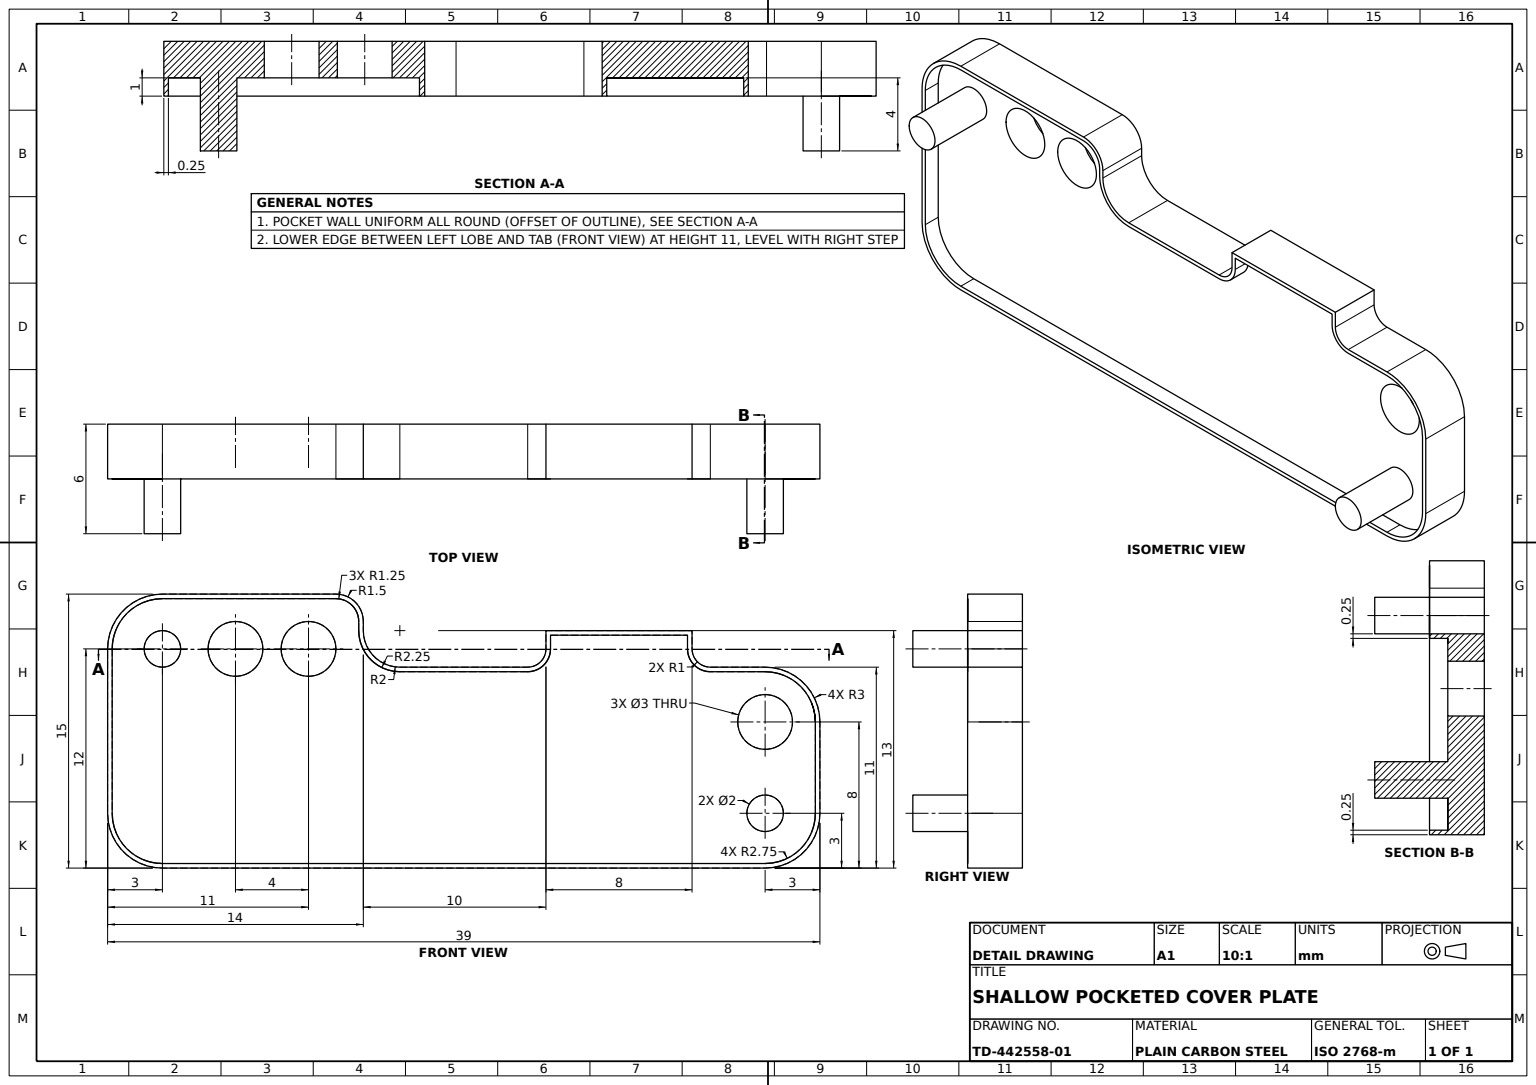
from build123d import *

# Parameters (mm, degrees)
PLATE_OUTLINE_SKETCH_R       = 1
PLATE_OUTLINE_SKETCH_R_2     = 1.5
BASE_PLATE_3MM_DEPTH         = 3
RECESS_POCKET_1MM_DEPTH      = 22.106870919
RECESS_POCKET_1MM_DEPTH_BACK = 1
LOCATING_PIN_SKETCH_R        = 1
LOCATING_PINS_2X_DEPTH       = 6


with BuildPart() as part:
    # Plate Outline Sketch → Base Plate 3mm (new body)
    with BuildSketch(Plane.XY):
        with BuildLine():
            Line((4.5, 5.5), (12.5, 5.5))
            Line((12.5, 5.5), (12.5, 4.5))
            ThreePointArc((12.5, 4.5), (12.792893219, 3.792893219), (13.5, 3.5))
            Line((13.5, 3.5), (16.5, 3.5))
            ThreePointArc((16.5, 3.5), (18.621320344, 2.621320344), (19.5, 0.5))
            Line((19.5, 0.5), (19.5, -4.5))
            ThreePointArc((19.5, -4.5), (18.621320344, -6.621320344), (16.5, -7.5))
            Line((16.5, -7.5), (-16.5, -7.5))
            ThreePointArc((-16.5, -7.5), (-18.621320344, -6.621320344), (-19.5, -4.5))
            Line((-19.5, -4.5), (-19.5, 4.5))
            ThreePointArc((-19.5, 4.5), (-18.621320344, 6.621320344), (-16.5, 7.5))
            Line((-16.5, 7.5), (-7, 7.5))
            ThreePointArc((-7, 7.5), (-5.939339828, 7.060660172), (-5.5, 6))
            Line((-5.5, 6), (-5.5, 5.5))
            ThreePointArc((-5.5, 5.5), (-4.914213562, 4.085786438), (-3.5, 3.5))
            Line((-3.5, 3.5), (3.5, 3.5))
            ThreePointArc((3.5, 3.5), (4.207106781, 3.792893219), (4.5, 4.5))
            Line((4.5, 4.5), (4.5, 5.5))
        make_face()
        with Locations((-16.5, 4.5)):
            Circle(PLATE_OUTLINE_SKETCH_R, mode=Mode.SUBTRACT)
        with Locations((-12.5, 4.5)):
            Circle(PLATE_OUTLINE_SKETCH_R_2, mode=Mode.SUBTRACT)
        with Locations((-8.5, 4.5)):
            Circle(PLATE_OUTLINE_SKETCH_R_2, mode=Mode.SUBTRACT)
        with Locations((16.5, 0.5)):
            Circle(PLATE_OUTLINE_SKETCH_R_2, mode=Mode.SUBTRACT)
        with Locations((16.5, -4.5)):
            Circle(PLATE_OUTLINE_SKETCH_R, mode=Mode.SUBTRACT)
    extrude(amount=BASE_PLATE_3MM_DEPTH)

    # Pocket Outline Sketch → Recess Pocket 1mm (cut, two sides: drawn at the far end of the back side and taken through both)
    with BuildSketch(Plane.XY.offset(3).offset(-RECESS_POCKET_1MM_DEPTH_BACK)):
        with BuildLine():
            Line((16.5, 3.25), (13.5, 3.25))
            ThreePointArc((13.5, 3.25), (12.616116524, 3.616116524), (12.25, 4.5))
            Line((12.25, 4.5), (12.25, 5.25))
            Line((12.25, 5.25), (4.75, 5.25))
            Line((4.75, 5.25), (4.75, 4.5))
            ThreePointArc((4.75, 4.5), (4.383883476, 3.616116524), (3.5, 3.25))
            Line((3.5, 3.25), (-3.5, 3.25))
            ThreePointArc((-3.5, 3.25), (-5.090990258, 3.909009742), (-5.75, 5.5))
            Line((-5.75, 5.5), (-5.75, 6))
            ThreePointArc((-5.75, 6), (-6.116116524, 6.883883476), (-7, 7.25))
            Line((-7, 7.25), (-16.5, 7.25))
            ThreePointArc((-16.5, 7.25), (-18.444543648, 6.444543648), (-19.25, 4.5))
            Line((-19.25, 4.5), (-19.25, -4.5))
            ThreePointArc((-19.25, -4.5), (-18.444543648, -6.444543648), (-16.5, -7.25))
            Line((-16.5, -7.25), (16.5, -7.25))
            ThreePointArc((16.5, -7.25), (18.444543648, -6.444543648), (19.25, -4.5))
            Line((19.25, -4.5), (19.25, 0.5))
            ThreePointArc((19.25, 0.5), (18.444543648, 2.444543648), (16.5, 3.25))
        make_face()
    extrude(amount=RECESS_POCKET_1MM_DEPTH + RECESS_POCKET_1MM_DEPTH_BACK, mode=Mode.SUBTRACT)

    # Locating Pin Sketch → Locating Pins 2x (add)
    with BuildSketch(Plane(origin=(0, 0, 0), x_dir=(-1, 0, 0), z_dir=(0, 0, -1))):
        with Locations((16.5, 4.5)):
            Circle(LOCATING_PIN_SKETCH_R)
        with Locations((-16.5, -4.5)):
            Circle(LOCATING_PIN_SKETCH_R)
    extrude(amount=-LOCATING_PINS_2X_DEPTH)


solid = part.part
